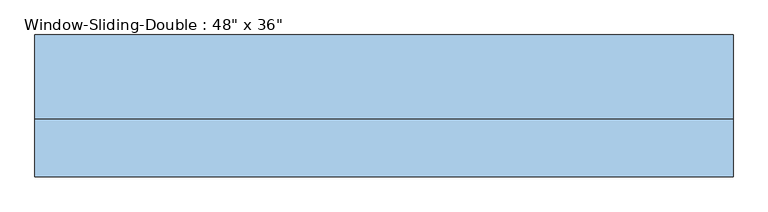
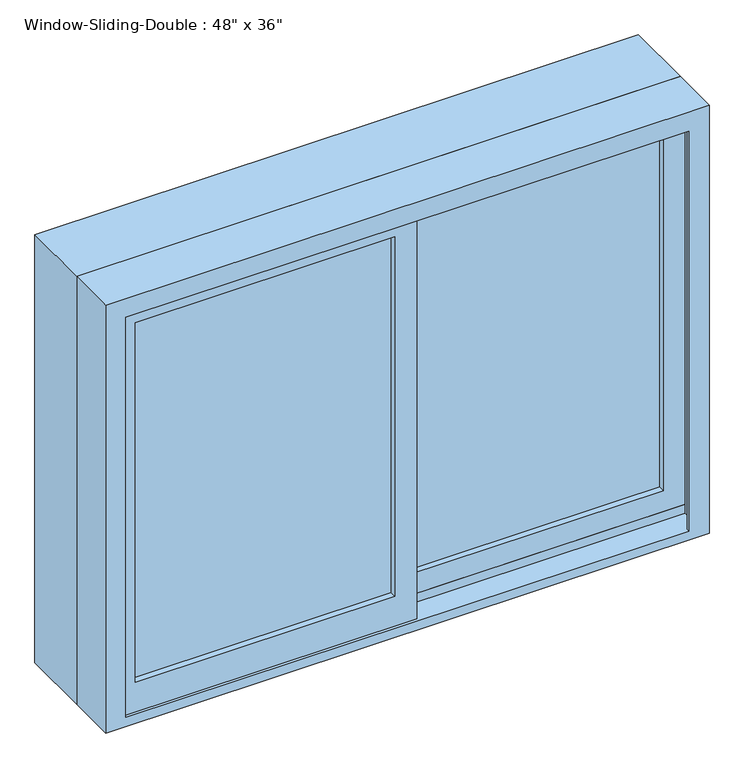
"""IFC4 building model written with IfcOpenShell, lengths in millimetres: window geometry."""

from ifc_helpers import new_model, si_unit, frame, origin, place, context, project, spatial, polyline, outline, extrude, faceted_brep, source, transform, mapped, element, save


def window_a5b1ea32(model_context):
    return source(origin(), model_context, "Body", "SolidModel", [
        extrude(outline(polyline([(952.5, -22.225), (952.5, 590.55), (1809.75, 590.55), (1809.75, -22.225), (952.5, -22.225)]), holes=[polyline([(996.95, 546.1), (996.95, 22.225), (1765.3, 22.225), (1765.3, 546.1), (996.95, 546.1)])]), frame((0.0, -78.74, 0.0), z_axis=(0.0, 1.0, 0.0), x_axis=(0.0, 0.0, 1.0)), (0.0, 0.0, 1.0), 44.45),
        extrude(outline(polyline([(933.45, 22.225), (1809.75, 22.225), (1809.75, -590.55), (933.45, -590.55), (933.45, 22.225)]), holes=[polyline([(1765.3, -546.1), (1765.3, -22.225), (996.95, -22.225), (996.95, -546.1), (1765.3, -546.1)])]), frame((0.0, -123.19, 0.0), z_axis=(0.0, 1.0, 0.0), x_axis=(0.0, 0.0, 1.0)), (0.0, 0.0, 1.0), 44.45),
        extrude(outline(polyline([(-22.225, -110.49), (-546.1, -110.49), (-546.1, -104.14), (-22.225, -104.14), (-22.225, -110.49)])), frame((0.0, 0.0, 996.95), z_axis=(0.0, 0.0, 1.0), x_axis=(1.0, 0.0, 0.0)), (0.0, 0.0, 1.0), 768.35),
        extrude(outline(polyline([(-22.225, -97.79), (-546.1, -97.79), (-546.1, -91.44), (-22.225, -91.44), (-22.225, -97.79)])), frame((0.0, 0.0, 996.95), z_axis=(0.0, 0.0, 1.0), x_axis=(1.0, 0.0, 0.0)), (0.0, 0.0, 1.0), 768.35),
        extrude(outline(polyline([(546.1, -66.04), (22.225, -66.04), (22.225, -59.69), (546.1, -59.69), (546.1, -66.04)])), frame((0.0, 0.0, 996.95), z_axis=(0.0, 0.0, 1.0), x_axis=(1.0, 0.0, 0.0)), (0.0, 0.0, 1.0), 768.35),
        extrude(outline(polyline([(546.1, -53.34), (22.225, -53.34), (22.225, -46.99), (546.1, -46.99), (546.1, -53.34)])), frame((0.0, 0.0, 996.95), z_axis=(0.0, 0.0, 1.0), x_axis=(1.0, 0.0, 0.0)), (0.0, 0.0, 1.0), 768.35),
        extrude(outline(polyline([(1828.8, 609.6), (1828.8, -609.6), (914.4, -609.6), (914.4, 609.6), (1828.8, 609.6)]), holes=[polyline([(1809.75, -590.55), (1809.75, 590.55), (933.45, 590.55), (933.45, -590.55), (1809.75, -590.55)])]), frame((0.0, -27.94, 0.0), z_axis=(0.0, 1.0, 0.0), x_axis=(0.0, 0.0, 1.0)), (0.0, 0.0, 1.0), 146.05),
        faceted_brep([(-609.6, -27.94, 914.4), (609.6, -27.94, 914.4), (609.6, -129.54, 914.4), (-609.6, -129.54, 914.4), (-568.6778905, -129.54, 1787.8778905), (-568.6778905, -129.54, 933.45), (-568.6778905, -123.19, 933.45), (-568.6778905, -123.19, 1787.8778905), (-590.55, -123.19, 933.45), (-590.55, -123.19, 1809.75), (590.55, -123.19, 1809.75), (590.55, -123.19, 933.45), (568.6778905, -123.19, 933.45), (568.6778905, -123.19, 1787.8778905), (-590.55, -78.74, 933.45), (-590.55, -78.74, 952.5), (-590.55, -34.29, 952.5), (-590.55, -34.29, 933.45), (-590.55, -27.94, 933.45), (-590.55, -27.94, 1809.75), (-609.6, -27.94, 1828.8), (609.6, -27.94, 1828.8), (590.55, -27.94, 1809.75), (590.55, -27.94, 933.45), (-609.6, -129.54, 1828.8), (609.6, -129.54, 1828.8), (568.6778905, -129.54, 1787.8778905), (568.6778905, -129.54, 933.45), (590.55, -34.29, 933.45), (590.55, -34.29, 952.5), (590.55, -78.74, 952.5), (590.55, -78.74, 933.45)], [[[0, 1, 2, 3]], [[4, 5, 6, 7]], [[7, 6, 8, 9, 10, 11, 12, 13]], [[9, 8, 14, 15, 16, 17, 18, 19]], [[0, 20, 21, 1], [22, 19, 18, 23]], [[24, 20, 0, 3]], [[2, 25, 24, 3], [4, 26, 27, 5]], [[7, 13, 26, 4]], [[9, 19, 22, 10]], [[20, 24, 25, 21]], [[13, 12, 27, 26]], [[22, 23, 28, 29, 30, 31, 11, 10]], [[21, 25, 2, 1]], [[27, 12, 11, 31, 14, 8, 6, 5]], [[31, 30, 15, 14]], [[30, 29, 16, 15]], [[29, 28, 17, 16]], [[18, 17, 28, 23]]]),
    ])


if __name__ == "__main__":
    model = new_model("IFC4")
    model_context = context("Model", 3, world=origin())
    ifc_project = project(units=[si_unit("LENGTHUNIT", "METRE", prefix="MILLI")], contexts=[model_context])
    site = spatial("IfcSite", under=ifc_project)
    building = spatial("IfcBuilding", under=site)
    placement = place(None, origin())
    window_shape = window_a5b1ea32(model_context)
    element("IfcWindow", 1, ObjectType="Window-Sliding-Double : 48\" x 36\"", at=placement, inside=building, context=model_context, shape_type="MappedRepresentation", body=[
        mapped(window_shape, transform((0.0, 0.0, 0.0), x_axis=(1.0, 0.0, 0.0), y_axis=(0.0, 1.0, 0.0), z_axis=(0.0, 0.0, 1.0))),
    ])
    save(model, "model.ifc")

# Revit data of these elements
# Type "Window-Sliding-Double : 48\" x 36\""
#   Type Mark = "18"
#   Fire Rating = "0.5h"
#   Assembly Code = "B2020100"
#   Analytic Construction = "Double glazing - domestic"
#   Window Inset [instance default] = 0' - 0"
#   Wall Thickness [instance default] = 0' - 6"
#   Visual Light Transmittance = 0.81
#   Thermal Resistance (R) = 1.8146 (h·ft²·°F)/BTU
#   Solar Heat Gain Coefficient = 0.76
#   Muntin Width = 1' - 8 5/8"
#   Muntin Height = 2' - 6 1/4"
#   Interior Wall Closure [instance default] = 0' - 2 3/4"
#   Heat Transfer Coefficient (U) = 0.5511 BTU/(h·ft²·°F)
#   Frame Extension [instance default] = 0' - 0 1/4"
#   Exterior Wall Closure [instance default] = 0' - 1 1/4"
#   Rough Width = 4' - 0 1/2"
#   Rough Height = 3' - 0 1/2"
#   Height = 3' - 0"
#   Extension Jamb [instance default] = 0' - 2 3/4"
#   Default Sill Height = 3' - 0"
#   Width = 4' - 0"
#   Interior Trim Visibility [instance default] = yes
#   Indicator Visibility [instance default] = yes
#   Exterior Trim Visibility [instance default] = yes
#   Muntin Visibility = yes
#   Extension Jamb Visibility [instance default] = yes
#   Muntin Pattern = Muntin Pattern_2x2 : Muntin Pattern_2x2
#   Interior Trim Material = Wood - Stained
#   Interior Trim = Trim-Window-Interior-Flat : Picture Frame
#   Interior Frame Material = Wood - Stained
#   Glass Panel Material = Glass
#   Exterior Trim Material = Clad - White
#   Exterior Trim = Trim-Window-Exterior-Flat : with Sill
#   Exterior Frame Material = Clad - White
#   Wall Closure = (empty or 0)
# Element 1 (IfcWindow, "Window-Sliding-Double : 48\" x 36\"")
#   Wall Thickness = 0' - 9"
#   Extension Jamb = 0' - 5 3/4"
#   Materials on its faces: "Wood - Stained", "Glass", "Clad - White"
# Materials
#   "Wood - Stained": class "Wood", colour RGB 224 178 126, transparency 0, Cost = 0
#   "Glass": class "Glass", colour RGB 0 128 192, transparency 0.75, Description = "Soda Lime Glass", Cost = 0
#   "Clad - White": class "Wood", colour RGB 242 242 238, transparency 0, Cost = 0
